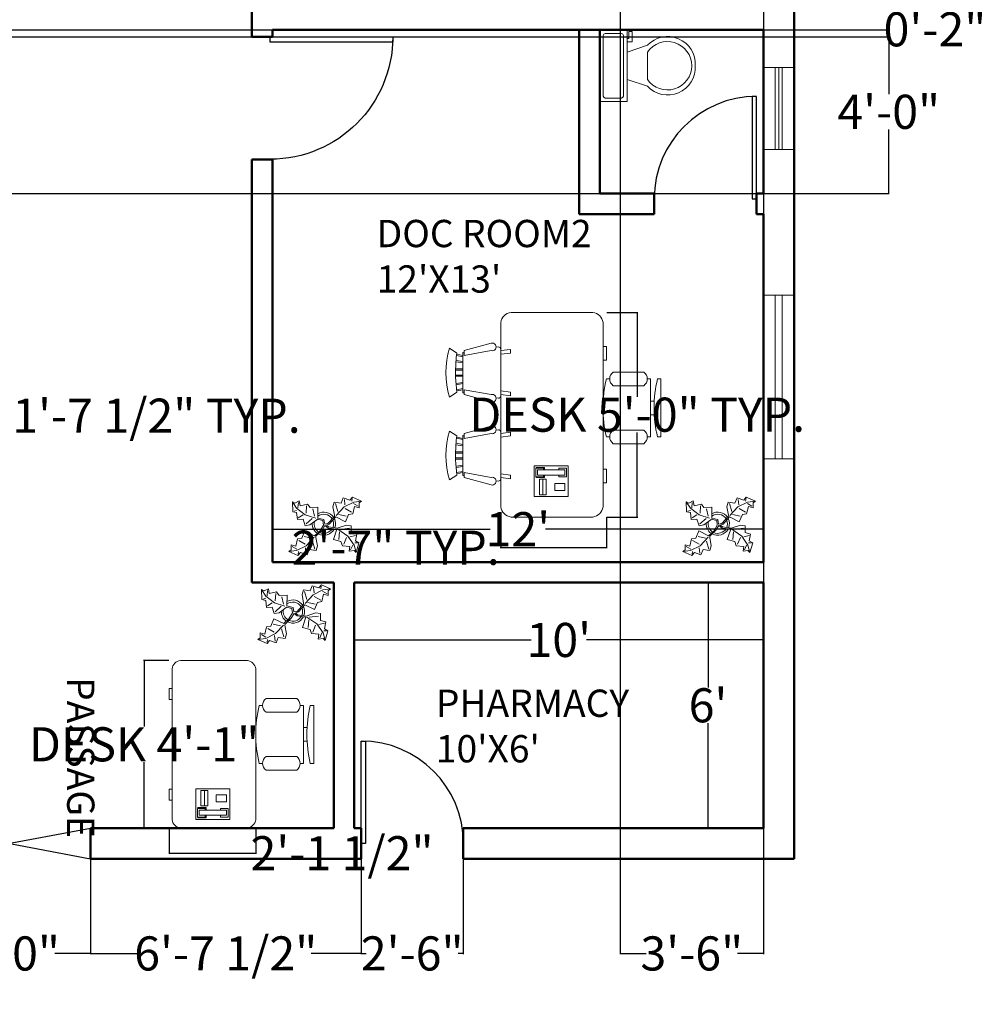
# Model space of a CAD drawing. Units: inches. Extents: x 69 to 644, y 258 to 887.
# Tile 2 of 3: x 335 to 619, y 258 to 546. Entities that reach past the tile are written whole.
import ezdxf

# ---------------------------------------------------------------- set-up
doc = ezdxf.new("R2010")
doc.units = ezdxf.units.IN
doc.header["$MEASUREMENT"] = 0
for name, color, linetype, lineweight in [('A-ANNO-DIMS', 2, 'Continuous', 18), ('A-AREA-IDEN', 7, 'Continuous', 25), ('A-DOOR', 4, 'Continuous', 25), ('A-EQPM', 8, 'Continuous', 13), ('A-FLOR-FIXT', 9, 'Continuous', 18), ('A-FURN', 8, 'Continuous', 18), ('A-GLAZ', 4, 'Continuous', 18), ('A-WALL', 7, 'Continuous', 50), ('PLANT', 3, 'Continuous', 13)]:
    doc.layers.add(name, color=color, linetype=linetype, lineweight=lineweight)
doc.styles.get("Standard").update_dxf_attribs({"font": 'arial.ttf'})
doc.dimstyles.get("Standard").update_dxf_attribs({"dimtxt": 10, "dimasz": 0.18, "dimexe": 0.18, "dimexo": 0.0625, "dimgap": 0.09, "dimtad": 0, "dimtih": 1, "dimtoh": 1, "dimdec": 0, "dimzin": 0, "dimdsep": 46, "dimlunit": 3, "dimtxsty": 'Standard', "dimcen": 0.09, "dimadec": 0, "dimazin": 0, "dimtfac": 1, "dimtdec": 0, "dimtofl": 0, "dimtmove": 0, "dimatfit": 3, "dimfxl": 1, "dimtolj": 1, "dimtzin": 0, "dimarcsym": 0})

# ---------------------------------------------------------------- blocks, each defined once
blk = doc.blocks.new('Desk - 30 x 60 in.')
for p, q in [((-26.999995, 0), (26.999995, 0)), ((-29.999995, -27), (-29.999995, -3)), ((29.999995, -3), (29.999995, -27)), ((26.999995, -30), (-26.999995, -30)), ((-20.000005, -30), (-20.000005, -31)), ((-20.000005, -31), (-16.000005, -31)), ((-16.000005, -31), (-16.000005, -30)), ((15.999995, -31), (15.999995, -30)), ((19.999995, -31), (15.999995, -31)), ((19.999995, -30), (19.999995, -31))]:
    blk.add_line(p, q)
for centre, start, end in [((-26.499995, -3.5), 98.1301, 171.8699), ((26.499995, -3.5), 8.130102, 81.8699), ((-26.499995, -26.5), 188.1301, 261.8699), ((26.499995, -26.5), 278.1301, 351.8699)]:
    blk.add_arc(centre, 3.535534, start, end)
blk = doc.blocks.new('Chair - Desk')
for p, q in [((-8.5, 0), (-8.5, -1)), ((-8.5, 0), (8.5, 0)), ((8.5, 0), (8.5, -1)), ((-2, -3), (-2, -1.9355)), ((2, -1.9576), (2, -3)), ((-10.5, -5), (-10.5, -14)), ((-8.5, -3), (-8.5, -4)), ((-8.5, -3), (8.5, -3)), ((-6.5, -14), (-6.5, -5)), ((6.5, -5), (6.5, -14)), ((8.5, -3), (8.5, -4)), ((10.5, -14), (10.5, -5)), ((-8.5, -15), (-8.5, -16)), ((8.5, -15), (8.5, -16))]:
    blk.add_line(p, q)
for centre, radius, start, end in [((0, 34.625), 36.625, 256.5803, 283.4197), ((-8.5, -6.5), 2.5, 36.8699, 143.1301), ((8.5, -6.5), 2.5, 36.8699, 143.1301), ((-8.5, -12.5), 2.5, 216.8699, 323.1301), ((8.5, -12.5), 2.5, 216.8699, 323.1301), ((0, 19.625), 36.625, 256.5803, 283.4197)]:
    blk.add_arc(centre, radius, start, end)
blk = doc.blocks.new('Phone - Desk')
for p, q in [((-4.5, -5), (-4.5, 5)), ((-4.5, 5), (4.5, 5)), ((-4, 4.5), (-4, 2)), ((-3.75, 4.5), (-3.75, 2.25)), ((-1.25, 4.5), (-3.75, 4.5)), ((-3.25, 4), (-3.25, -4)), ((-3.25, 4), (-1.75, 4)), ((-1.75, -4), (-1.75, 4)), ((-1.25, 2.25), (-1.25, 4.5)), ((-1, 2), (-1, 4.5)), ((4, 3.5), (-0.5, 3.5)), ((-0.5, 3.5), (-0.5, 1.5)), ((4, 1.5), (4, 3.5)), ((4.5, 5), (4.5, -5)), ((-4, 2), (-3.25, 2)), ((-3.75, 2.25), (-3.25, 2.25)), ((-1.75, 2.25), (-1.25, 2.25)), ((-1.75, 2), (-1, 2)), ((-0.5, 2.5), (4, 2.5)), ((-0.5, 1.5), (4, 1.5)), ((-3.75, -2.25), (-3.25, -2.25)), ((-3.75, -4.5), (-3.75, -2.25)), ((-1.75, -2.25), (-1.25, -2.25)), ((-1.25, -2.25), (-1.25, -4.5)), ((2.75, -1), (0.75, -1)), ((0.75, -1), (0.75, -4)), ((2.75, -4), (2.75, -1)), ((4.5, -5), (-4.5, -5)), ((-1.25, -4.5), (-3.75, -4.5)), ((-3.25, -4), (-1.75, -4)), ((0.75, -4), (2.75, -4))]:
    blk.add_line(p, q)
blk = doc.blocks.new('Chair - Rocking')
for p, q in [((-8, -4.5), (-10, -1.5)), ((8, -4.5), (10, -1.5)), ((-9, -7.5), (-12, -18.49999)), ((-7, -7.5), (-9, -7.5)), ((-9, -18.49999), (-7, -7.5)), ((-8.23428, -6.99939), (-8.3093, -7.47958)), ((-8.23041, -7), (8.23915, -7)), ((-7.5, -4.5), (-7, -7)), ((-6.5, -7), (-7.02225, -4.43)), ((-4.5, -7), (-4.96674, -4.19951)), ((-4, -7), (-4.40532, -4.16272)), ((-1.5, -4.05012), (-1.5, -7)), ((-1, -7), (-1, -4.05012)), ((1, -7), (1, -4.04655)), ((1.5, -4.05012), (1.5, -7)), ((4, -7), (4.40187, -4.18694)), ((4.5, -7), (4.96761, -4.19437)), ((6.5, -7), (7, -4.4057)), ((7.5, -4.5), (7, -7)), ((7, -7.5), (9, -7.5)), ((9, -18.49999), (7, -7.5)), ((8.31071, -7.48854), (8.23449, -7.00073)), ((9, -7.5), (12, -18.49999)), ((-10.36644, -20.64523), (-10.5, -21.49999)), ((-9, -22.49999), (-9.5, -26.49999)), ((0, -22.49999), (-9.5, -22.49999)), ((-8, -26.49999), (-7.5, -22.49999)), ((0, -22.49999), (9.5, -22.49999)), ((8, -26.49999), (7.5, -22.49999)), ((9, -22.49999), (9.5, -26.49999)), ((10.5, -21.49999), (10.3575, -20.58798)), ((-9.5, -26.49999), (-8, -26.49999)), ((9.5, -26.49999), (8, -26.49999))]:
    blk.add_line(p, q)
for centre, radius, start, end in [((0, -34.08333), 34.08333, 72.93847, 107.0615), ((0, -68.25004), 64.25, 82.84733, 93.92211), ((0, -68.25004), 64.25, 93.92211, 97.15267), ((-10.5, -18.99999), 1.58114, 161.5651, 18.43495), ((10.5, -18.99999), 1.58114, 161.5651, 18.43495), ((-9.5, -21.49999), 1, 180, 270), ((9.5, -21.49999), 1, 270, 0)]:
    blk.add_arc(centre, radius, start, end)
blk = doc.blocks.new('Plant - Rubber or Philodendron')
for p, q in [((-16.2005, 11.4774), (-13.9899, 8.1064)), ((-16.2005, 11.4774), (-14.8639, 10.7964)), ((-16.0159, 6.3329), (-16.2005, 11.4774)), ((-14.8639, 10.7964), (-12.6195, 11.8975)), ((-13.3174, 8.325), (-13.0735, 11.0065)), ((-12.6195, 11.8975), (-12.1909, 9.4345)), ((-12.1909, 9.4345), (-8.3829, 10.3)), ((-8.3829, 10.3), (-7.0549, 8.501)), ((4.6914, 8.8812), (5.3859, 11.2828)), ((5.3859, 11.2828), (8.8871, 10.7908)), ((5.9878, 10.4842), (7.1971, 6.3869)), ((8.8871, 10.7908), (9.9809, 13.4933)), ((9.9809, 13.4933), (13.3837, 12.301)), ((15.3859, 11.3055), (10.3916, 8.7942)), ((10.5828, 12.6946), (10.8893, 9.7953)), ((13.3837, 12.301), (14.68, 13.9039)), ((14.5816, 13.2037), (14.3848, 11.8033)), ((14.68, 13.9039), (19.3848, 11.8146)), ((15.2875, 10.6053), (17.5907, 9.2105)), ((19.3848, 11.8146), (15.3859, 11.3055)), ((19.3848, 11.8146), (18.1868, 10.9119)), ((18.1868, 10.9119), (18.1925, 8.4119)), ((-14.0069, 5.8704), (-16.0159, 6.3329)), ((-15.3434, 6.5514), (-13.9984, 6.9884)), ((-13.5868, 2.2894), (-14.0069, 5.8704)), ((-13.9899, 8.1064), (-9.5434, 4.7185)), ((-8.8369, 9.409), (-9.0894, 5.6095)), ((-7.0549, 8.501), (-3.0284, 8.6941)), ((-4.8529, 4.012), (-5.7184, 7.82)), ((-3.0284, 8.6941), (-3.0709, 3.1041)), ((4.6914, 8.8812), (5.5014, 4.4831)), ((10.3916, 8.7942), (6.2847, 4.4028)), ((14.2977, 6.1031), (10.9934, 7.9956)), ((14.8995, 5.3044), (12.7005, 4.8994)), ((15.7909, 9.1065), (14.8995, 5.3044)), ((18.1925, 8.4119), (15.7909, 9.1065)), ((-10.6784, 2.491), (-13.5868, 2.2894)), ((-13.1329, 3.1804), (-10.6614, 4.727)), ((-9.5858, -0.8715), (-10.6784, 2.491)), ((-9.5434, 4.7185), (-4.1917, 2.9888)), ((-9.1318, 0.0195), (-5.9793, 2.9025)), ((-7.1228, -0.443), (-3.5248, 2.2131)), ((-3.5248, 2.2131), (-3.3011, 2.4355)), ((-3.3011, 2.4355), (-0.5306, 1.7947)), ((-3.0709, 3.1041), (0.0797, 2.3163)), ((-0.5306, 1.7947), (-0.2255, -0.5527)), ((-0.5306, 1.7947), (-0.5306, 1.7947)), ((0.0797, 2.3163), (0.4866, -0.031)), ((0.4866, -0.031), (2.1141, 0.2298)), ((2.1141, 0.2298), (5.4346, 3.9146)), ((6.1032, 3.6844), (2.8262, -0.031)), ((5.4346, 3.9146), (5.5014, 4.4831)), ((11.1089, 1.1958), (6.1032, 3.6844)), ((7.7005, 4.8881), (11.5025, 3.9967)), ((12.7005, 4.8994), (11.1089, 1.1958)), ((-11.3237, -7.2629), (-9.7321, -3.5593)), ((-9.7321, -3.5593), (-4.7264, -6.0479)), ((-7.1228, -0.443), (-9.5858, -0.8715)), ((-2.019, -3.6148), (-4.7264, -6.0479)), ((-4.0579, -6.2781), (-0.9375, -3.1608)), ((-2.019, -3.6148), (-0.2255, -0.5527)), ((-0.9375, -3.1608), (0.5883, -0.8135)), ((0.5883, -0.8135), (2.2447, -2.0916)), ((2.8262, -0.031), (1.3003, -0.5527)), ((1.3003, -0.5527), (2.4193, -1.4655)), ((2.2447, -2.0916), (6.7108, -2.6626)), ((2.4193, -1.4655), (6.895, -2.1175)), ((4.943, -7.9659), (6.7108, -2.6626)), ((11.6605, -0.5413), (6.895, -2.1175)), ((12.3677, -6.1981), (7.219, -2.6772)), ((8.125, -4.0768), (7.7715, -7.9659)), ((8.3544, -2.7453), (13.1973, -2.1704)), ((11.6605, -0.5413), (14.1354, -0.8948)), ((14.1354, -0.8948), (14.1354, -4.4304)), ((14.1354, -4.4304), (16.9638, -5.1375)), ((-14.4141, -11.4699), (-13.5228, -7.6679)), ((-13.5228, -7.6679), (-11.3237, -7.2629)), ((-12.921, -8.4665), (-9.6166, -10.359)), ((-6.3237, -7.2516), (-10.1257, -6.3602)), ((-9.0148, -11.1577), (-4.9047, -6.8122)), ((-4.611, -12.8477), (-5.8203, -8.7504)), ((-4.1246, -6.8466), (-4.0579, -6.2781)), ((-3.3146, -11.2447), (-4.1246, -6.8466)), ((8.8321, -9.0266), (4.943, -7.9659)), ((9.5392, -11.1479), (8.8321, -9.0266)), ((10.2463, -10.4408), (11.6605, -6.9053)), ((15.5496, -10.7943), (12.3677, -6.1981)), ((16.2567, -5.8446), (13.4283, -6.5517)), ((17.3174, -9.7337), (15.9032, -9.7337)), ((16.9638, -5.1375), (16.2567, -8.673)), ((16.2567, -8.673), (18.0245, -9.7337)), ((18.0245, -9.7337), (16.6103, -14.6834)), ((-18.008, -14.1781), (-16.8101, -13.2754)), ((-18.008, -14.1781), (-14.0091, -13.669)), ((-13.3032, -16.2674), (-18.008, -14.1781)), ((-16.8157, -10.7754), (-14.4141, -11.4699)), ((-16.8101, -13.2754), (-16.8157, -10.7754)), ((-13.9107, -12.9688), (-16.2139, -11.574)), ((-14.0091, -13.669), (-9.0148, -11.1577)), ((-12.0069, -14.6645), (-13.3032, -16.2674)), ((-13.2048, -15.5672), (-13.008, -14.1668)), ((-8.6042, -15.8568), (-12.0069, -14.6645)), ((-9.206, -15.0581), (-9.5126, -12.1588)), ((-7.5103, -13.1543), (-8.6042, -15.8568)), ((-4.0092, -13.6463), (-7.5103, -13.1543)), ((-3.3146, -11.2447), (-4.0092, -13.6463)), ((13.4283, -11.5015), (9.5392, -11.1479)), ((13.0748, -13.9763), (13.4283, -11.5015)), ((15.5496, -13.6228), (13.0748, -13.9763)), ((14.8425, -10.7943), (13.7819, -13.2692)), ((16.6103, -14.6834), (15.5496, -10.7943)), ((16.6103, -14.6834), (15.5496, -13.6228))]:
    blk.add_line(p, q)
for centre, radius, start, end in [((0, 0), 6.1275, 34.37569, 120.1028), ((0.0308, 0.1664), 6, 178.6147, 235.1169), ((0.0308, 0.1664), 5, 168.1647, 238.6725), ((-0.0601, -0.2075), 5.2461, 33.82192, 124.9414), ((-0.2664, 0.1682), 5.2775, 338.4094, 20.03007), ((-0.098, 0.1364), 6.1288, 341.2017, 26.09184), ((-0.0234, 0.3825), 6.1492, 242.5812, 331.2714), ((-0.1102, 0.4886), 5.2883, 247.3711, 327.472)]:
    blk.add_arc(centre, radius, start, end)
blk = doc.blocks.new('*U15')
for p, q in [((0, 0), (0, -6)), ((-40, 0), (-40, -6))]:
    blk.add_line(p, q)
blk.add_lwpolyline([(0, 0), (0, 40), (-1.75, 40), (-1.75, 0)], close=True)
blk.add_arc((0, 0), 40, 90, 180)
blk = doc.blocks.new('*U17')
for p, q in [((9.5, -6), (9.5, -2)), ((-10, -8.5), (-8, -8.5)), ((-10, -9.5), (-10, -8.5)), ((-8, -8.5), (-8, -8)), ((-7, -8), (-7, -9.5)), ((-4, -8), (-6, -14)), ((4, -8), (6, -14)), ((-7, -9.5), (-10, -9.5)), ((4, -14), (-4, -14))]:
    blk.add_line(p, q)
blk.add_lwpolyline([(10.5, -8), (10.5, 0), (-10.5, 0), (-10.5, -8)], close=True)
for points in [[(-9.5, -2), (-9.5, -6)], [(8.5, -1), (-8.5, -1)], [(-8.5, -7), (8.5, -7)]]:
    blk.add_lwpolyline(points)
for centre, radius, start, end in [((-8.625, -1.875), 0.8839, 81.8699, 188.1301), ((8.625, -1.875), 0.8839, 351.8699, 98.1301), ((-8.625, -6.125), 0.8839, 171.869898, 278.1301), ((8.625, -6.125), 0.8839, 261.8699, 8.1301), ((-0.4772, -19.9188), 8.0953, 133.01722, 273.38), ((0.0374, -19.8731), 7.127, 124.50543, 269.7), ((-0.0373, -19.8731), 7.127, 270.3, 55.4946), ((0.4773, -19.9188), 8.0953, 266.62, 46.9828)]:
    blk.add_arc(centre, radius, start, end)
blk = doc.blocks.new('*U14')
for p, q in [((0, 0), (0, -6)), ((40, 0), (40, -6))]:
    blk.add_line(p, q)
blk.add_lwpolyline([(0, 0), (0, 40), (1.75, 40), (1.75, 0)], close=True)
blk.add_arc((0, 0), 40, 0, 90)
blk = doc.blocks.new('*D23')
at = {"layer": 'A-ANNO-DIMS', "color": 0, "lineweight": -2, "transparency": 16777216}
for p, q in [((409.27, 387.48), (409.27, 397.22)), ((409.45, 397.04), (473.16, 397.04)), ((553.09, 397.04), (489.37, 397.04)), ((553.27, 387.48), (553.27, 397.22))]:
    blk.add_line(p, q, dxfattribs=at)
at = {"layer": 'A-ANNO-DIMS', "color": 0, "transparency": 16777216}
for points in [[(409.45, 397.07), (409.45, 397.01), (409.27, 397.04)], [(553.09, 397.07), (553.09, 397.01), (553.27, 397.04)]]:
    blk.add_solid(points, dxfattribs=at)
at = {"layer": 'Defpoints', "color": 0, "transparency": 16777216}
for p in [(553.27, 397.04), (409.27, 387.42), (553.27, 387.42)]:
    blk.add_point(p, dxfattribs=at)
at = {"layer": 'A-ANNO-DIMS', "color": 0, "transparency": 16777216, "insert": (481.27, 397.04), "char_height": 10, "attachment_point": 5}
blk.add_mtext("\\A1;12'", dxfattribs=at)
blk = doc.blocks.new('*D24')
at = {"layer": 'A-ANNO-DIMS', "color": 0, "lineweight": -2, "transparency": 16777216}
for p, q in [((553.2, 381.42), (536.85, 381.42)), ((537.03, 381.24), (537.03, 350.62)), ((537.03, 309.6), (537.03, 340.22)), ((553.2, 309.42), (536.85, 309.42))]:
    blk.add_line(p, q, dxfattribs=at)
at = {"layer": 'A-ANNO-DIMS', "color": 0, "transparency": 16777216}
for points in [[(537, 381.24), (537.06, 381.24), (537.03, 381.42)], [(537, 309.6), (537.06, 309.6), (537.03, 309.42)]]:
    blk.add_solid(points, dxfattribs=at)
at = {"layer": 'Defpoints', "color": 0, "transparency": 16777216}
for p in [(553.27, 381.42), (537.03, 309.42), (553.27, 309.42)]:
    blk.add_point(p, dxfattribs=at)
at = {"layer": 'A-ANNO-DIMS', "color": 0, "transparency": 16777216, "insert": (537.03, 345.42), "char_height": 10, "attachment_point": 5}
blk.add_mtext("\\A1;6'", dxfattribs=at)
blk = doc.blocks.new('*D25')
at = {"layer": 'A-ANNO-DIMS', "color": 0, "lineweight": -2, "transparency": 16777216}
for p, q in [((433.27, 381.36), (433.27, 364.4)), ((553.27, 381.18), (553.27, 364.4)), ((433.45, 364.58), (485.16, 364.58)), ((553.09, 364.58), (501.37, 364.58))]:
    blk.add_line(p, q, dxfattribs=at)
at = {"layer": 'A-ANNO-DIMS', "color": 0, "transparency": 16777216}
for points in [[(433.45, 364.61), (433.45, 364.55), (433.27, 364.58)], [(553.09, 364.61), (553.09, 364.55), (553.27, 364.58)]]:
    blk.add_solid(points, dxfattribs=at)
at = {"layer": 'Defpoints', "color": 0, "transparency": 16777216}
for p in [(433.27, 381.42), (553.27, 381.24), (553.27, 364.58)]:
    blk.add_point(p, dxfattribs=at)
at = {"layer": 'A-ANNO-DIMS', "color": 0, "transparency": 16777216, "insert": (493.27, 364.58), "char_height": 10, "attachment_point": 5}
blk.add_mtext("\\A1;10'", dxfattribs=at)
blk = doc.blocks.new('WIN-48IN')
for p, q in [((9, 48), (0, 48)), ((3.5, 0), (3.5, 48)), ((5.5, 0), (5.5, 48)), ((9, 0), (0, 0))]:
    blk.add_line(p, q)
blk = doc.blocks.new('WIN-24IN')
for p, q in [((0, 0), (0, 9)), ((24, 0), (24, 9)), ((0, 5.5), (24, 5.5)), ((0, 4.5), (24, 4.5)), ((0, 3.5), (24, 3.5))]:
    blk.add_line(p, q)
blk = doc.blocks.new('*D35')
at = {"layer": 'A-ANNO-DIMS', "color": 0, "lineweight": -2, "transparency": 16777216}
for p, q in [((219.29, 427.48), (219.29, 430.5)), ((219.47, 430.32), (238.47, 430.32)), ((238.65, 427.48), (238.65, 430.5)), ((238.65, 430.32), (238.83, 430.32))]:
    blk.add_line(p, q, dxfattribs=at)
at = {"layer": 'A-ANNO-DIMS', "color": 0, "transparency": 16777216}
for points in [[(219.47, 430.35), (219.47, 430.29), (219.29, 430.32)], [(238.47, 430.35), (238.47, 430.29), (238.65, 430.32)]]:
    blk.add_solid(points, dxfattribs=at)
at = {"layer": 'Defpoints', "color": 0, "transparency": 16777216}
for p in [(238.65, 430.32), (219.29, 427.41), (238.65, 427.41)]:
    blk.add_point(p, dxfattribs=at)
at = {"layer": 'A-ANNO-DIMS', "color": 0, "transparency": 16777216, "insert": (330.64, 430.32), "char_height": 10, "attachment_point": 5}
blk.add_mtext('\\A1;GUEST CHAIR 1\'-7 1/2" TYP.', dxfattribs=at)
blk = doc.blocks.new('*D41')
at = {"layer": 'A-ANNO-DIMS', "color": 0, "lineweight": -2, "transparency": 16777216}
for p, q in [((378.95, 358.55), (371.46, 358.55)), ((371.64, 358.37), (371.64, 339.25)), ((371.64, 309.6), (371.64, 328.72)), ((378.95, 309.42), (371.46, 309.42))]:
    blk.add_line(p, q, dxfattribs=at)
at = {"layer": 'A-ANNO-DIMS', "color": 0, "transparency": 16777216}
for points in [[(371.61, 358.37), (371.67, 358.37), (371.64, 358.55)], [(371.61, 309.6), (371.67, 309.6), (371.64, 309.42)]]:
    blk.add_solid(points, dxfattribs=at)
at = {"layer": 'Defpoints', "color": 0, "transparency": 16777216}
for p in [(379.01, 358.55), (371.64, 309.42), (379.01, 309.42)]:
    blk.add_point(p, dxfattribs=at)
at = {"layer": 'A-ANNO-DIMS', "color": 0, "transparency": 16777216, "insert": (371.64, 333.98), "char_height": 10, "attachment_point": 5}
blk.add_mtext('\\A1;DESK 4\'-1"', dxfattribs=at)
blk = doc.blocks.new('*D42')
at = {"layer": 'A-ANNO-DIMS', "color": 0, "lineweight": -2, "transparency": 16777216}
for p, q in [((379.01, 309.36), (379.01, 301.87)), ((404.4, 309.36), (404.4, 301.87)), ((379.19, 302.05), (404.22, 302.05)), ((404.4, 302.05), (404.58, 302.05))]:
    blk.add_line(p, q, dxfattribs=at)
at = {"layer": 'A-ANNO-DIMS', "color": 0, "transparency": 16777216}
for points in [[(379.19, 302.08), (379.19, 302.02), (379.01, 302.05)], [(404.22, 302.08), (404.22, 302.02), (404.4, 302.05)]]:
    blk.add_solid(points, dxfattribs=at)
at = {"layer": 'Defpoints', "color": 0, "transparency": 16777216}
for p in [(379.01, 309.42), (404.4, 309.42), (404.4, 302.05)]:
    blk.add_point(p, dxfattribs=at)
at = {"layer": 'A-ANNO-DIMS', "color": 0, "transparency": 16777216, "insert": (429.69, 302.05), "char_height": 10, "attachment_point": 5}
blk.add_mtext('\\A1;2\'-1 1/2"', dxfattribs=at)
blk = doc.blocks.new('*D43')
at = {"layer": 'A-ANNO-DIMS', "color": 0, "lineweight": -2, "transparency": 16777216}
for p, q in [((507.32, 460.62), (516.44, 460.62)), ((516.26, 460.44), (516.26, 435.89)), ((516.26, 400.8), (516.26, 425.36)), ((507.32, 400.62), (516.44, 400.62))]:
    blk.add_line(p, q, dxfattribs=at)
at = {"layer": 'A-ANNO-DIMS', "color": 0, "transparency": 16777216}
for points in [[(516.23, 460.44), (516.29, 460.44), (516.26, 460.62)], [(516.23, 400.8), (516.29, 400.8), (516.26, 400.62)]]:
    blk.add_solid(points, dxfattribs=at)
at = {"layer": 'Defpoints', "color": 0, "transparency": 16777216}
for p in [(507.26, 460.62), (507.26, 400.62), (516.26, 400.62)]:
    blk.add_point(p, dxfattribs=at)
at = {"layer": 'A-ANNO-DIMS', "color": 0, "transparency": 16777216, "insert": (516.26, 430.62), "char_height": 10, "attachment_point": 5}
blk.add_mtext('\\A1;DESK 5\'-0" TYP.', dxfattribs=at)
blk = doc.blocks.new('*D44')
at = {"layer": 'A-ANNO-DIMS', "color": 0, "lineweight": -2, "transparency": 16777216}
for p, q in [((476.26, 400.56), (476.26, 391.44)), ((507.26, 400.56), (507.26, 391.44)), ((476.26, 391.62), (476.08, 391.62)), ((507.08, 391.62), (476.44, 391.62))]:
    blk.add_line(p, q, dxfattribs=at)
at = {"layer": 'A-ANNO-DIMS', "color": 0, "transparency": 16777216}
for points in [[(476.44, 391.65), (476.44, 391.59), (476.26, 391.62)], [(507.08, 391.65), (507.08, 391.59), (507.26, 391.62)]]:
    blk.add_solid(points, dxfattribs=at)
at = {"layer": 'Defpoints', "color": 0, "transparency": 16777216}
for p in [(476.26, 400.62), (507.26, 400.62), (476.26, 391.62)]:
    blk.add_point(p, dxfattribs=at)
at = {"layer": 'A-ANNO-DIMS', "color": 0, "transparency": 16777216, "insert": (445.43, 391.62), "char_height": 10, "attachment_point": 5}
blk.add_mtext('\\A1;2\'-7" TYP.', dxfattribs=at)
blk = doc.blocks.new('*D54')
at = {"layer": 'A-ANNO-DIMS', "color": 0, "lineweight": -2, "transparency": 16777216}
for p, q in [((307.91, 300.36), (307.91, 272.49)), ((355.91, 300.36), (355.91, 272.49)), ((308.09, 272.67), (318.33, 272.67)), ((355.73, 272.67), (345.49, 272.67))]:
    blk.add_line(p, q, dxfattribs=at)
at = {"layer": 'A-ANNO-DIMS', "color": 0, "transparency": 16777216}
for points in [[(308.09, 272.7), (308.09, 272.64), (307.91, 272.67)], [(355.73, 272.7), (355.73, 272.64), (355.91, 272.67)]]:
    blk.add_solid(points, dxfattribs=at)
at = {"layer": 'Defpoints', "color": 0, "transparency": 16777216}
for p in [(307.91, 300.42), (355.91, 300.42), (355.91, 272.67)]:
    blk.add_point(p, dxfattribs=at)
at = {"layer": 'A-ANNO-DIMS', "color": 0, "transparency": 16777216, "insert": (331.91, 272.67), "char_height": 10, "attachment_point": 5}
blk.add_mtext('\\A1;4\'-0"', dxfattribs=at)
blk = doc.blocks.new('*D55')
at = {"layer": 'A-ANNO-DIMS', "color": 0, "lineweight": -2, "transparency": 16777216}
for p, q in [((355.91, 300.36), (355.91, 272.49)), ((435.27, 300.36), (435.27, 272.49)), ((356.09, 272.67), (370.53, 272.67)), ((435.09, 272.67), (420.65, 272.67))]:
    blk.add_line(p, q, dxfattribs=at)
at = {"layer": 'A-ANNO-DIMS', "color": 0, "transparency": 16777216}
for points in [[(356.09, 272.7), (356.09, 272.64), (355.91, 272.67)], [(435.09, 272.7), (435.09, 272.64), (435.27, 272.67)]]:
    blk.add_solid(points, dxfattribs=at)
at = {"layer": 'Defpoints', "color": 0, "transparency": 16777216}
for p in [(355.91, 300.42), (435.27, 300.42), (435.27, 272.67)]:
    blk.add_point(p, dxfattribs=at)
at = {"layer": 'A-ANNO-DIMS', "color": 0, "transparency": 16777216, "insert": (395.59, 272.67), "char_height": 10, "attachment_point": 5}
blk.add_mtext('\\A1;6\'-7 1/2"', dxfattribs=at)
blk = doc.blocks.new('*D56')
at = {"layer": 'A-ANNO-DIMS', "color": 0, "lineweight": -2, "transparency": 16777216}
for p, q in [((435.27, 300.36), (435.27, 272.49)), ((465.27, 300.36), (465.27, 272.49)), ((435.45, 272.67), (436.8, 272.67)), ((465.09, 272.67), (463.73, 272.67))]:
    blk.add_line(p, q, dxfattribs=at)
at = {"layer": 'A-ANNO-DIMS', "color": 0, "transparency": 16777216}
for points in [[(435.45, 272.7), (435.45, 272.64), (435.27, 272.67)], [(465.09, 272.7), (465.09, 272.64), (465.27, 272.67)]]:
    blk.add_solid(points, dxfattribs=at)
at = {"layer": 'Defpoints', "color": 0, "transparency": 16777216}
for p in [(435.27, 300.42), (465.27, 300.42), (465.27, 272.67)]:
    blk.add_point(p, dxfattribs=at)
at = {"layer": 'A-ANNO-DIMS', "color": 0, "transparency": 16777216, "insert": (450.27, 272.67), "char_height": 10, "attachment_point": 5}
blk.add_mtext('\\A1;2\'-6"', dxfattribs=at)
blk = doc.blocks.new('*D60')
at = {"layer": 'A-ANNO-DIMS', "color": 0, "lineweight": -2, "transparency": 16777216}
for p, q in [((199.33, 543.42), (590.2, 543.42)), ((590.02, 543.24), (590.02, 524.62)), ((590.02, 495.6), (590.02, 514.22)), ((199.33, 495.42), (590.2, 495.42))]:
    blk.add_line(p, q, dxfattribs=at)
at = {"layer": 'A-ANNO-DIMS', "color": 0, "transparency": 16777216}
for points in [[(589.99, 543.24), (590.05, 543.24), (590.02, 543.42)], [(589.99, 495.6), (590.05, 495.6), (590.02, 495.42)]]:
    blk.add_solid(points, dxfattribs=at)
at = {"layer": 'Defpoints', "color": 0, "transparency": 16777216}
for p in [(199.27, 543.42), (199.27, 495.42), (590.02, 495.42)]:
    blk.add_point(p, dxfattribs=at)
at = {"layer": 'A-ANNO-DIMS', "color": 0, "transparency": 16777216, "insert": (590.02, 519.42), "char_height": 10, "attachment_point": 5}
blk.add_mtext('\\A1;4\'-0"', dxfattribs=at)
blk = doc.blocks.new('*D66')
at = {"layer": 'A-ANNO-DIMS', "color": 0, "lineweight": -2, "transparency": 16777216}
for p, q in [((511.27, 735.36), (511.27, 272.49)), ((553.27, 735.36), (553.27, 272.49)), ((511.45, 272.67), (518.89, 272.67)), ((553.09, 272.67), (545.64, 272.67))]:
    blk.add_line(p, q, dxfattribs=at)
at = {"layer": 'A-ANNO-DIMS', "color": 0, "transparency": 16777216}
for points in [[(511.45, 272.7), (511.45, 272.64), (511.27, 272.67)], [(553.09, 272.7), (553.09, 272.64), (553.27, 272.67)]]:
    blk.add_solid(points, dxfattribs=at)
at = {"layer": 'Defpoints', "color": 0, "transparency": 16777216}
for p in [(511.27, 735.42), (553.27, 735.42), (553.27, 272.67)]:
    blk.add_point(p, dxfattribs=at)
at = {"layer": 'A-ANNO-DIMS', "color": 0, "transparency": 16777216, "insert": (532.27, 272.67), "char_height": 10, "attachment_point": 5}
blk.add_mtext('\\A1;3\'-6"', dxfattribs=at)
blk = doc.blocks.new('*D70')
at = {"layer": 'A-ANNO-DIMS', "color": 0, "lineweight": -2, "transparency": 16777216}
for p, q in [((295.33, 543.42), (590.2, 543.42)), ((590.02, 543.42), (590.02, 543.6)), ((590.02, 543.6), (590.2, 543.6)), ((590.02, 541.6), (590.02, 543.24)), ((295.33, 541.42), (590.2, 541.42))]:
    blk.add_line(p, q, dxfattribs=at)
at = {"layer": 'A-ANNO-DIMS', "color": 0, "transparency": 16777216}
for points in [[(589.99, 543.24), (590.05, 543.24), (590.02, 543.42)], [(589.99, 541.6), (590.05, 541.6), (590.02, 541.42)]]:
    blk.add_solid(points, dxfattribs=at)
at = {"layer": 'Defpoints', "color": 0, "transparency": 16777216}
for p in [(295.27, 543.42), (590.02, 543.42), (295.27, 541.42)]:
    blk.add_point(p, dxfattribs=at)
at = {"layer": 'A-ANNO-DIMS', "color": 0, "transparency": 16777216, "insert": (603.58, 543.6), "char_height": 10, "attachment_point": 5}
blk.add_mtext('\\A1;0\'-2"', dxfattribs=at)

msp = doc.modelspace()

# ---------------------------------------------------------------- linework, layer by layer
at = {"layer": 'A-DOOR'}
for p, q in [((307.91, 309.42), (355.91, 300.42)), ((307.91, 300.42), (355.91, 309.42))]:
    msp.add_line(p, q, dxfattribs=at)
at = {"layer": 'A-WALL'}
for p, q in [((562.27, 852.42), (562.27, 300.42)), ((403.27, 549.42), (403.27, 543.42)), ((403.27, 543.42), (403.27, 541.42)), ((409.27, 543.42), (553.27, 543.42)), ((409.27, 541.42), (409.27, 543.42)), ((499.27, 543.42), (499.27, 489.42)), ((505.27, 543.42), (505.27, 495.42)), ((553.27, 543.42), (553.27, 495.42)), ((403.27, 541.42), (409.27, 541.42)), ((403.27, 505.42), (409.27, 505.42)), ((403.27, 505.42), (403.27, 381.42)), ((409.27, 505.42), (409.27, 387.42)), ((505.27, 495.42), (521.27, 495.42)), ((521.27, 495.42), (521.27, 489.42)), ((553.27, 495.42), (551.27, 495.42)), ((551.27, 495.42), (551.27, 489.42)), ((499.27, 489.42), (521.27, 489.42)), ((551.27, 489.42), (553.27, 489.42)), ((553.27, 489.42), (553.27, 387.42)), ((553.27, 387.42), (409.27, 387.42)), ((427.27, 381.42), (403.27, 381.42)), ((427.27, 381.42), (427.27, 309.42)), ((553.27, 381.42), (433.27, 381.42)), ((433.27, 381.42), (433.27, 309.42)), ((553.27, 381.42), (553.27, 309.42)), ((355.91, 309.42), (355.91, 300.42)), ((427.27, 309.42), (355.91, 309.42)), ((435.27, 309.42), (433.27, 309.42)), ((435.27, 300.42), (435.27, 309.42)), ((553.27, 309.42), (465.27, 309.42)), ((465.27, 309.42), (465.27, 300.42)), ((433.27, 300.42), (355.91, 300.42)), ((433.27, 300.42), (435.27, 300.42)), ((562.27, 300.42), (465.27, 300.42))]:
    msp.add_line(p, q, dxfattribs=at)

# ---------------------------------------------------------------- block references
at = {"layer": 'A-DOOR', "xscale": -0.8980321148011755, "yscale": 0.8980321148011755, "zscale": 0.8980321148011755, "rotation": 270}
msp.add_blockref('*U15', (408.65, 541.42), dxfattribs=at)
at = {"layer": 'A-DOOR'}
for name, p, xscale, yscale, zscale in [('*U15', (551.27, 493.92), 0.7503359922981823, 0.7503359922981823, 0.7503359922981823), ('*U14', (435.27, 304.92), 0.7506699854318816, 0.7506699854318816, 0.7506699854318816)]:
    msp.add_blockref(name, p, dxfattribs=dict(at, xscale=xscale, yscale=yscale, zscale=zscale))
at = {"layer": 'A-EQPM', "xscale": -1, "rotation": 90}
msp.add_blockref('Phone - Desk', (491.06, 411.17), dxfattribs=at)
at = {"layer": 'A-EQPM', "rotation": 90}
msp.add_blockref('Phone - Desk', (391.82, 316.41), dxfattribs=at)
at = {"layer": 'A-FLOR-FIXT', "xscale": -1, "rotation": 90}
msp.add_blockref('*U17', (505.27, 532.91), dxfattribs=at)
at = {"layer": 'A-FURN', "xscale": -1}
for name, p, rotation in [('Desk - 30 x 60 in.', (476.26, 430.62), 90), ('Chair - Desk', (523.21, 432.62), 270)]:
    msp.add_blockref(name, p, dxfattribs=dict(at, rotation=rotation))
at = {"layer": 'A-FURN'}
for name, p, xscale, yscale, zscale, rotation in [('Chair - Rocking', (460.13, 442.95), -0.716801753801156, 0.716801753801156, 0.716801753801156, 90), ('Chair - Rocking', (460.13, 418.66), -0.716801753801156, 0.716801753801156, 0.716801753801156, 90), ('Desk - 30 x 60 in.', (404.4, 333.98), 0.8188455003231441, 0.8188455003231441, 0.8188455003231441, 270)]:
    msp.add_blockref(name, p, dxfattribs=dict(at, xscale=xscale, yscale=yscale, zscale=zscale, rotation=rotation))
at = {"layer": 'A-FURN', "rotation": 270}
msp.add_blockref('Chair - Desk', (421.4, 336.9), dxfattribs=at)
at = {"layer": 'A-GLAZ'}
for name, p, rotation in [('WIN-24IN', (562.27, 508.41), 89.99999999999982), ('WIN-48IN', (562.27, 465.63), 180)]:
    msp.add_blockref(name, p, dxfattribs=dict(at, rotation=rotation))
at = {"layer": 'PLANT', "xscale": 0.5698547619027642, "yscale": 0.5698547619027642, "zscale": 0.5698547619027642}
for p in [(424.36, 398.56), (539.87, 398.56), (415.29, 372.8)]:
    msp.add_blockref('Plant - Rubber or Philodendron', p, dxfattribs=at)

# ---------------------------------------------------------------- texts
at = {"layer": 'A-AREA-IDEN', "char_height": 8, "attachment_point": 1}
for s, width, heights, insert in [("DOC ROOM2\\P12'X13'", 77.0373, [44.4], (439.85, 487.73)), ("PHARMACY\\P10'X6'", 64.3137, [0], (457.22, 350.02))]:
    msp.add_mtext_dynamic_manual_height_columns(s, width=width, gutter_width=1, heights=heights, dxfattribs=dict(at, insert=insert))
at = {"layer": 'A-AREA-IDEN', "insert": (357.08, 353.68), "char_height": 8, "attachment_point": 1, "rotation": 270}
msp.add_mtext_dynamic_manual_height_columns('PASSAGE', width=64.3137, gutter_width=1, heights=[0], dxfattribs=at)

# ---------------------------------------------------------------- dimensions: what is measured, and where the dimension line sits
at = {"layer": 'A-ANNO-DIMS'}
for base, p1, p2, override, picture, middle in [((553.27, 272.67), (511.27, 735.42), (553.27, 735.42), {"dimdec": 1, "dimlfac": 1, "dimrnd": 0, "dimzin": 1, "dimdsep": 46, "dimlunit": 4, "dimfrac": 2}, '*D66', (532.27, 272.67)), ((553.27, 397.04), (409.27, 387.42), (553.27, 387.42), {"dimclrd": 0, "dimclre": 0, "dimclrt": 0}, '*D23', (481.27, 397.04)), ((553.27, 364.58), (433.27, 381.42), (553.27, 381.24), {"dimclrd": 0, "dimclre": 0, "dimclrt": 0}, '*D25', (493.27, 364.58)), ((404.4, 302.05), (379.01, 309.42), (404.4, 309.42), {"dimdec": 1, "dimlfac": 1, "dimrnd": 0, "dimzin": 1, "dimdsep": 46, "dimlunit": 4, "dimfrac": 2}, '*D42', (429.69, 302.05)), ((355.91, 272.67), (307.91, 300.42), (355.91, 300.42), {"dimdec": 1, "dimlfac": 1, "dimrnd": 0, "dimzin": 1, "dimdsep": 46, "dimlunit": 4, "dimfrac": 2}, '*D54', (331.91, 272.67)), ((435.27, 272.67), (355.91, 300.42), (435.27, 300.42), {"dimdec": 1, "dimlfac": 1, "dimrnd": 0, "dimzin": 1, "dimdsep": 46, "dimlunit": 4, "dimfrac": 2}, '*D55', (395.59, 272.67)), ((465.27, 272.67), (435.27, 300.42), (465.27, 300.42), {"dimdec": 1, "dimlfac": 1, "dimrnd": 0, "dimzin": 1, "dimdsep": 46, "dimlunit": 4, "dimfrac": 2}, '*D56', (450.27, 272.67))]:
    dim = msp.add_linear_dim(base=base, p1=p1, p2=p2, dimstyle='Standard', override=override, dxfattribs=at)
    dim.commit()
    dim.dimension.update_dxf_attribs({"geometry": picture, "text_midpoint": middle})
for base, p1, p2, override, picture, middle in [((590.02, 543.42), (295.27, 541.42), (295.27, 543.42), {"dimdec": 1, "dimlfac": 1, "dimrnd": 0, "dimzin": 1, "dimdsep": 46, "dimlunit": 4, "dimfrac": 2}, '*D70', (603.58, 543.6)), ((590.02, 495.42), (199.27, 543.42), (199.27, 495.42), {"dimdec": 1, "dimlfac": 1, "dimrnd": 0, "dimzin": 1, "dimdsep": 46, "dimlunit": 4, "dimfrac": 2}, '*D60', (590.02, 519.42)), ((537.03, 309.42), (553.27, 381.42), (553.27, 309.42), {"dimclrd": 0, "dimclre": 0, "dimclrt": 0}, '*D24', (537.03, 345.42))]:
    dim = msp.add_linear_dim(base=base, p1=p1, p2=p2, angle=90, dimstyle='Standard', override=override, dxfattribs=at)
    dim.commit()
    dim.dimension.update_dxf_attribs({"geometry": picture, "text_midpoint": middle})
dim = msp.add_linear_dim(base=(238.65, 430.32), p1=(219.29, 427.41), p2=(238.65, 427.41), text='GUEST CHAIR <> TYP.', dimstyle='Standard', override={"dimdec": 1, "dimlfac": 1, "dimrnd": 0, "dimzin": 1, "dimdsep": 46, "dimlunit": 4, "dimfrac": 2}, dxfattribs=at)
dim.commit()
dim.dimension.update_dxf_attribs({"geometry": '*D35', "text_midpoint": (330.64, 430.32)})
for base, p1, p2, angle, text, picture, middle in [((516.26, 400.62), (507.26, 460.62), (507.26, 400.62), 270, 'DESK <> TYP.', '*D43', (516.26, 430.62)), ((476.26, 391.62), (507.26, 400.62), (476.26, 400.62), 180, '<> TYP.', '*D44', (445.43, 391.62)), ((371.64, 309.42), (379.01, 358.55), (379.01, 309.42), 270, 'DESK <>', '*D41', (371.64, 333.98))]:
    dim = msp.add_linear_dim(base=base, p1=p1, p2=p2, angle=angle, text=text, dimstyle='Standard', override={"dimdec": 1, "dimlfac": 1, "dimrnd": 0, "dimzin": 1, "dimdsep": 46, "dimlunit": 4, "dimfrac": 2}, dxfattribs=at)
    dim.commit()
    dim.dimension.update_dxf_attribs({"geometry": picture, "text_midpoint": middle})

doc.saveas('drawing.dxf')
